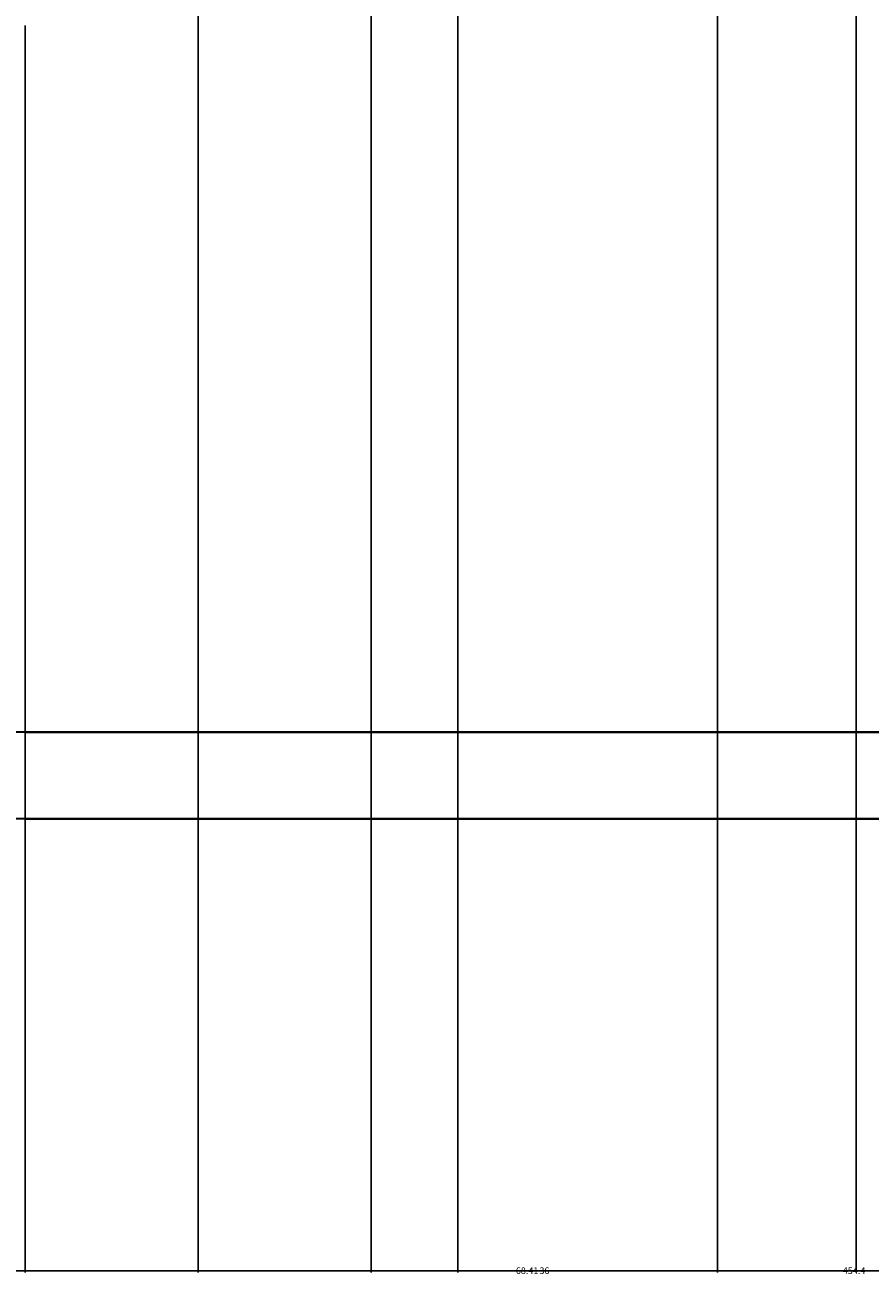
# Model space of a CAD drawing. Units: inches. Extents: x 867 to 1667, y -234 to 788.
# Tile 14 of 42: x 1212 to 1300, y -234 to -104. Entities that reach past the tile are written whole.
import ezdxf

# ---------------------------------------------------------------- set-up
doc = ezdxf.new("R2010")
doc.units = ezdxf.units.IN
doc.header["$MEASUREMENT"] = 0
doc.layers.add('A-ANNO-DIMS', color=2, linetype='Continuous', lineweight=18)
doc.layers.add('A-WALL-SITE', color=8, linetype='Continuous', lineweight=30)
doc.styles.get("Standard").update_dxf_attribs({"font": 'arial.ttf'})
doc.dimstyles.get("Standard").update_dxf_attribs({"dimtxt": 0.6875, "dimasz": 0.18, "dimexe": 0.18, "dimexo": 0.0625, "dimgap": 0.09, "dimtad": 0, "dimdec": 4, "dimzin": 0, "dimdsep": 46, "dimlunit": 4, "dimtxsty": 'Standard', "dimcen": 0.09, "dimadec": 0, "dimazin": 0, "dimtfac": 1, "dimtdec": 4, "dimtofl": 0, "dimtmove": 0, "dimatfit": 3, "dimfxl": 1, "dimtolj": 1, "dimtzin": 0, "dimarcsym": 0})

# ---------------------------------------------------------------- blocks, each defined once
blk = doc.blocks.new('*D27')
at = {"layer": 'A-ANNO-DIMS', "color": 0, "lineweight": -2, "transparency": 16777216}
for p, q in [((1070.89, -55.97), (1070.89, -233.54)), ((1525.26, -186.47), (1525.26, -233.54)), ((1071.07, -233.36), (1296.81, -233.36)), ((1525.08, -233.36), (1299.34, -233.36))]:
    blk.add_line(p, q, dxfattribs=at)
at = {"layer": 'A-ANNO-DIMS', "color": 0, "transparency": 16777216}
for points in [[(1071.07, -233.33), (1071.07, -233.39), (1070.89, -233.36)], [(1525.08, -233.33), (1525.08, -233.39), (1525.26, -233.36)]]:
    blk.add_solid(points, dxfattribs=at)
at = {"layer": 'Defpoints', "color": 0, "transparency": 16777216}
for p in [(1070.89, -55.91), (1525.26, -186.41), (1525.26, -233.36)]:
    blk.add_point(p, dxfattribs=at)
at = {"layer": 'A-ANNO-DIMS', "color": 0, "transparency": 16777216, "insert": (1298.08, -233.36), "char_height": 0.688, "attachment_point": 5}
blk.add_mtext('\\A1;454.4', dxfattribs=at)
blk = doc.blocks.new('*D30')
at = {"layer": 'A-ANNO-DIMS', "color": 0, "lineweight": -2, "transparency": 16777216}
for p, q in [((1229.89, 623.55), (1229.89, -233.54)), ((1298.3, 623.55), (1298.3, -233.54)), ((1230.07, -233.36), (1262.91, -233.36)), ((1298.12, -233.36), (1265.28, -233.36))]:
    blk.add_line(p, q, dxfattribs=at)
at = {"layer": 'A-ANNO-DIMS', "color": 0, "transparency": 16777216}
for points in [[(1230.07, -233.33), (1230.07, -233.39), (1229.89, -233.36)], [(1298.12, -233.33), (1298.12, -233.39), (1298.3, -233.36)]]:
    blk.add_solid(points, dxfattribs=at)
at = {"layer": 'Defpoints', "color": 0, "transparency": 16777216}
for p in [(1229.89, 623.62), (1298.3, 623.62), (1298.3, -233.36)]:
    blk.add_point(p, dxfattribs=at)
at = {"layer": 'A-ANNO-DIMS', "color": 0, "transparency": 16777216, "insert": (1264.09, -233.36), "char_height": 0.688, "attachment_point": 5}
blk.add_mtext('\\A1;68.41', dxfattribs=at)
blk = doc.blocks.new('*D45')
at = {"layer": 'A-ANNO-DIMS', "color": 0, "lineweight": -2, "transparency": 16777216}
for p, q in [((1079.89, -7.95), (1079.89, -233.54)), ((1247.89, -7.95), (1247.89, -233.54)), ((1080.07, -233.36), (1163.07, -233.36)), ((1247.71, -233.36), (1164.7, -233.36))]:
    blk.add_line(p, q, dxfattribs=at)
at = {"layer": 'A-ANNO-DIMS', "color": 0, "transparency": 16777216}
for points in [[(1080.07, -233.33), (1080.07, -233.39), (1079.89, -233.36)], [(1247.71, -233.33), (1247.71, -233.39), (1247.89, -233.36)]]:
    blk.add_solid(points, dxfattribs=at)
at = {"layer": 'Defpoints', "color": 0, "transparency": 16777216}
for p in [(1079.89, -7.88), (1247.89, -7.88), (1247.89, -233.36)]:
    blk.add_point(p, dxfattribs=at)
at = {"layer": 'A-ANNO-DIMS', "color": 0, "transparency": 16777216, "insert": (1163.89, -233.36), "char_height": 0.688, "attachment_point": 5}
blk.add_mtext('\\A1;168', dxfattribs=at)
blk = doc.blocks.new('*D46')
at = {"layer": 'A-ANNO-DIMS', "color": 0, "lineweight": -2, "transparency": 16777216}
for p, q in [((1256.89, -16.95), (1256.89, -233.54)), ((1394.89, -16.95), (1394.89, -233.54)), ((1257.07, -233.36), (1325.07, -233.36)), ((1394.71, -233.36), (1326.7, -233.36))]:
    blk.add_line(p, q, dxfattribs=at)
at = {"layer": 'A-ANNO-DIMS', "color": 0, "transparency": 16777216}
for points in [[(1257.07, -233.33), (1257.07, -233.39), (1256.89, -233.36)], [(1394.71, -233.33), (1394.71, -233.39), (1394.89, -233.36)]]:
    blk.add_solid(points, dxfattribs=at)
at = {"layer": 'Defpoints', "color": 0, "transparency": 16777216}
for p in [(1256.89, -16.88), (1394.89, -16.88), (1394.89, -233.36)]:
    blk.add_point(p, dxfattribs=at)
at = {"layer": 'A-ANNO-DIMS', "color": 0, "transparency": 16777216, "insert": (1325.89, -233.36), "char_height": 0.688, "attachment_point": 5}
blk.add_mtext('\\A1;138', dxfattribs=at)
blk = doc.blocks.new('*D48')
at = {"layer": 'A-ANNO-DIMS', "color": 0, "lineweight": -2, "transparency": 16777216}
for p, q in [((1283.89, -55.97), (1283.89, -233.54)), ((1355.89, -55.97), (1355.89, -233.54)), ((1284.07, -233.36), (1319.31, -233.36)), ((1355.71, -233.36), (1320.46, -233.36))]:
    blk.add_line(p, q, dxfattribs=at)
at = {"layer": 'A-ANNO-DIMS', "color": 0, "transparency": 16777216}
for points in [[(1284.07, -233.33), (1284.07, -233.39), (1283.89, -233.36)], [(1355.71, -233.33), (1355.71, -233.39), (1355.89, -233.36)]]:
    blk.add_solid(points, dxfattribs=at)
at = {"layer": 'Defpoints', "color": 0, "transparency": 16777216}
for p in [(1283.89, -55.91), (1355.89, -55.91), (1355.89, -233.36)]:
    blk.add_point(p, dxfattribs=at)
at = {"layer": 'A-ANNO-DIMS', "color": 0, "transparency": 16777216, "insert": (1319.89, -233.36), "char_height": 0.688, "attachment_point": 5}
blk.add_mtext('\\A1;72', dxfattribs=at)
blk = doc.blocks.new('*D50')
at = {"layer": 'A-ANNO-DIMS', "color": 0, "lineweight": -2, "transparency": 16777216}
for p, q in [((1211.89, -103.97), (1211.89, -233.54)), ((1427.89, -103.97), (1427.89, -233.54)), ((1212.07, -233.36), (1319.03, -233.36)), ((1427.71, -233.36), (1320.74, -233.36))]:
    blk.add_line(p, q, dxfattribs=at)
at = {"layer": 'A-ANNO-DIMS', "color": 0, "transparency": 16777216}
for points in [[(1212.07, -233.33), (1212.07, -233.39), (1211.89, -233.36)], [(1427.71, -233.33), (1427.71, -233.39), (1427.89, -233.36)]]:
    blk.add_solid(points, dxfattribs=at)
at = {"layer": 'Defpoints', "color": 0, "transparency": 16777216}
for p in [(1211.89, -103.91), (1427.89, -103.91), (1427.89, -233.36)]:
    blk.add_point(p, dxfattribs=at)
at = {"layer": 'A-ANNO-DIMS', "color": 0, "transparency": 16777216, "insert": (1319.89, -233.36), "char_height": 0.688, "attachment_point": 5}
blk.add_mtext('\\A1;216', dxfattribs=at)
blk = doc.blocks.new('*D62')
at = {"layer": 'A-ANNO-DIMS', "color": 0, "lineweight": -2, "transparency": 16777216}
for p, q in [((1247.89, -55.97), (1247.89, -233.54)), ((1283.89, -55.97), (1283.89, -233.54)), ((1248.07, -233.36), (1265.3, -233.36)), ((1283.71, -233.36), (1266.47, -233.36))]:
    blk.add_line(p, q, dxfattribs=at)
at = {"layer": 'A-ANNO-DIMS', "color": 0, "transparency": 16777216}
for points in [[(1248.07, -233.33), (1248.07, -233.39), (1247.89, -233.36)], [(1283.71, -233.33), (1283.71, -233.39), (1283.89, -233.36)]]:
    blk.add_solid(points, dxfattribs=at)
at = {"layer": 'Defpoints', "color": 0, "transparency": 16777216}
for p in [(1247.89, -55.91), (1283.89, -55.91), (1247.89, -233.36)]:
    blk.add_point(p, dxfattribs=at)
at = {"layer": 'A-ANNO-DIMS', "color": 0, "transparency": 16777216, "insert": (1265.89, -233.36), "char_height": 0.688, "attachment_point": 5}
blk.add_mtext('\\A1;36', dxfattribs=at)

msp = doc.modelspace()

# ---------------------------------------------------------------- linework, layer by layer
at = {"layer": 'A-WALL-SITE'}
for p, q in [((1526.8389, -177.4081), (1006.3882, -177.4081)), ((1211.8866, -177.4081), (1427.8866, -177.4081)), ((1619.8866, -186.4081), (914.8866, -186.4081)), ((1211.8866, -186.4081), (1427.8866, -186.4081))]:
    msp.add_line(p, q, dxfattribs=at)

# ---------------------------------------------------------------- dimensions: what is measured, and where the dimension line sits
at = {"layer": 'A-ANNO-DIMS'}
for base, p1, p2, override, picture, middle in [((1298.2966, -233.3581), (1229.8866, 623.617), (1298.2966, 623.617), {"dimdec": 2, "dimlfac": 1, "dimrnd": 0, "dimzin": 0, "dimdsep": 46, "dimlunit": 2}, '*D30', (1264.0916, -233.3581)), ((1247.8866, -233.3581), (1079.8866, -7.883), (1247.8866, -7.883), {"dimdec": 0, "dimlfac": 1, "dimrnd": 0, "dimzin": 0, "dimdsep": 46, "dimlunit": 2}, '*D45', (1163.8866, -233.3581)), ((1394.8866, -233.3581), (1256.8866, -16.883), (1394.8866, -16.883), {"dimdec": 0, "dimlfac": 1, "dimrnd": 0, "dimzin": 0, "dimdsep": 46, "dimlunit": 2}, '*D46', (1325.8866, -233.3581)), ((1525.2648, -233.3581), (1070.8866, -55.9081), (1525.2648, -186.4081), {"dimdec": 1, "dimlfac": 1, "dimrnd": 0, "dimzin": 0, "dimdsep": 46, "dimlunit": 2}, '*D27', (1298.0757, -233.3581)), ((1247.8866, -233.3581), (1283.8866, -55.9081), (1247.8866, -55.9081), {"dimdec": 0, "dimlfac": 1, "dimrnd": 0, "dimzin": 0, "dimdsep": 46, "dimlunit": 2}, '*D62', (1265.8866, -233.3581)), ((1355.8866, -233.3581), (1283.8866, -55.9081), (1355.8866, -55.9081), {"dimdec": 0, "dimlfac": 1, "dimrnd": 0, "dimzin": 0, "dimdsep": 46, "dimlunit": 2}, '*D48', (1319.8866, -233.3581)), ((1427.8866, -233.3581), (1211.8866, -103.9081), (1427.8866, -103.9081), {"dimdec": 0, "dimlfac": 1, "dimrnd": 0, "dimzin": 0, "dimdsep": 46, "dimlunit": 2}, '*D50', (1319.8866, -233.3581))]:
    dim = msp.add_linear_dim(base=base, p1=p1, p2=p2, dimstyle='Standard', override=override, dxfattribs=at)
    dim.commit()
    dim.dimension.update_dxf_attribs({"geometry": picture, "text_midpoint": middle})

doc.saveas('drawing.dxf')
